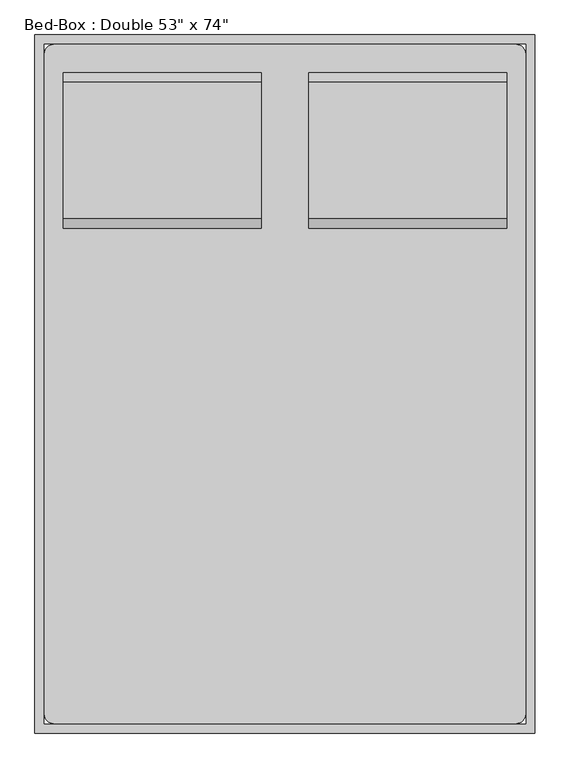
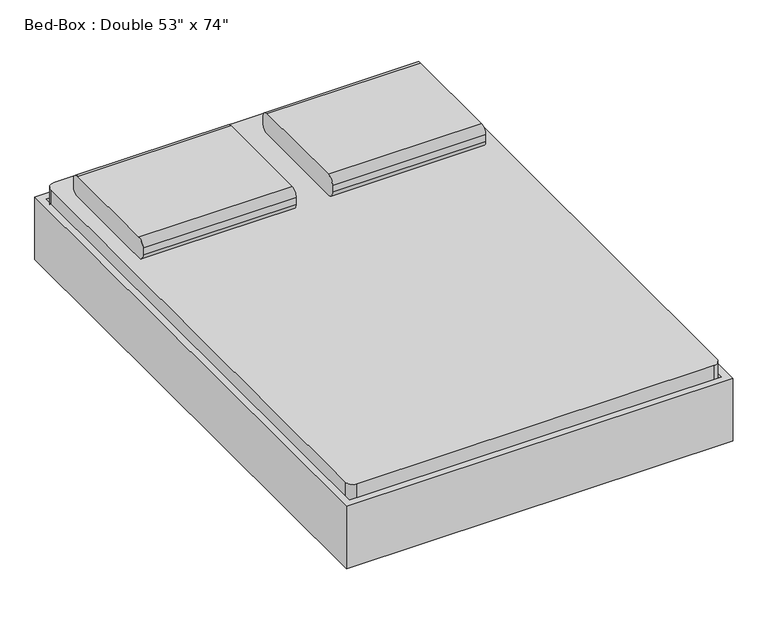
"""IFC4 building model written with IfcOpenShell, lengths in millimetres: furniture geometry."""

from ifc_helpers import new_model, si_unit, point, frame, frame_2d, origin, place, context, project, spatial, polyline, circle_curve, trimmed, segment, composite_curve, outline, extrude, source, transform, mapped, element, save
from ifc_brep_helpers import plane_surface, cylinder_surface, revolved_surface, advanced_brep


def furniture_b58f7881(model_context):
    return source(origin(), model_context, "Body", "SolidModel", [
        advanced_brep(
        [(-308.547541, -869.4295082, 196.85), (-308.547541, -869.4295082, 177.8), (-308.547541, -945.6295082, 177.8), (-308.547541, -945.6295082, 196.85), (-245.6113525, -869.4295082, 196.85), (-257.747541, -869.4295082, 177.8), (-257.747541, -945.6295082, 177.8), (-245.6113525, -945.6295082, 196.85), (-164.4115092, -869.4295082, 22.716374), (-181.6766725, -869.4295082, 14.6654962), (-181.6766725, -945.6295082, 14.6654962), (-164.4115092, -945.6295082, 22.716374), (-158.6564547, -869.4295082, 0.0), (-158.6564547, -869.4295082, 19.05), (-158.6564547, -945.6295082, 0.0), (-158.6564547, -945.6295082, 19.05), (-80.0439489, -869.4295082, 19.05), (-80.0439489, -869.4295082, 0.0), (-80.0439489, -945.6295082, 0.0), (-80.0439489, -945.6295082, 19.05), (-67.3439489, -869.4295082, 3.4029547), (-76.8689489, -869.4295082, 19.9007387), (-67.3439489, -945.6295082, 3.4029547), (-76.8689489, -945.6295082, 19.9007387), (-12.3513357, -869.4295082, 57.15), (-7.2469036, -869.4295082, 38.1), (-7.2469036, -945.6295082, 38.1), (-12.3513357, -945.6295082, 57.15), (690.6562537, -869.4295082, 57.15), (685.5518216, -869.4295082, 38.1), (685.5518216, -945.6295082, 38.1), (690.6562537, -945.6295082, 57.15), (755.1738669, -869.4295082, 19.9007387), (745.6488669, -869.4295082, 3.4029547), (745.6488669, -945.6295082, 3.4029547), (755.1738669, -945.6295082, 19.9007387), (758.3488669, -869.4295082, 0.0), (758.3488669, -869.4295082, 19.05), (758.3488669, -945.6295082, 0.0), (758.3488669, -945.6295082, 19.05), (836.9613728, -869.4295082, 19.05), (836.9613728, -869.4295082, 0.0), (836.9613728, -945.6295082, 0.0), (836.9613728, -945.6295082, 19.05), (859.9815906, -869.4295082, 14.6654962), (842.7164272, -869.4295082, 22.716374), (859.9815906, -945.6295082, 14.6654962), (842.7164272, -945.6295082, 22.716374), (923.9162705, -869.4295082, 196.85), (936.052459, -869.4295082, 177.8), (936.052459, -945.6295082, 177.8), (923.9162705, -945.6295082, 196.85), (986.852459, -869.4295082, 196.85), (986.852459, -945.6295082, 196.85), (986.852459, -945.6295082, 177.8), (986.852459, -869.4295082, 177.8)],
        [
            (0, 1),
            (1, 2),
            (2, 3),
            (3, 0),
            (0, 4),
            (4, 5),
            (5, 1),
            (5, 6),
            (6, 2),
            (6, 7),
            (7, 3),
            (7, 4),
            (4, 8),
            (8, 9),
            (9, 5),
            (9, 10),
            (10, 6),
            (10, 11),
            (11, 7),
            (11, 8),
            (12, 9, circle_curve(frame((-158.6564547, -869.4295082, 25.4), z_axis=(0.0, 1.0, 0.0), x_axis=(-0.906307787036663, 0.0, -0.4226182617406713)), 25.4)),
            (8, 13, circle_curve(frame((-158.6564547, -869.4295082, 25.4), z_axis=(0.0, -1.0, 0.0), x_axis=(-0.906307787036663, 0.0, -0.4226182617406713)), 6.35)),
            (13, 12),
            (14, 10, circle_curve(frame((-158.6564547, -945.6295082, 25.4), z_axis=(0.0, 1.0, 0.0), x_axis=(-0.906307787036663, 0.0, -0.4226182617406713)), 25.4)),
            (12, 14),
            (15, 11, circle_curve(frame((-158.6564547, -945.6295082, 25.4), z_axis=(0.0, 1.0, 0.0), x_axis=(-0.906307787036663, 0.0, -0.4226182617406713)), 6.35)),
            (14, 15),
            (15, 13),
            (13, 16),
            (16, 17),
            (17, 12),
            (17, 18),
            (18, 14),
            (18, 19),
            (19, 15),
            (19, 16),
            (20, 17, circle_curve(frame((-80.0439489, -869.4295082, 25.4), z_axis=(0.0, 1.0, 0.0), x_axis=(0.0, 0.0, -1.0)), 25.4)),
            (16, 21, circle_curve(frame((-80.0439489, -869.4295082, 25.4), z_axis=(0.0, -1.0, 0.0), x_axis=(0.0, 0.0, -1.0)), 6.35)),
            (21, 20),
            (22, 18, circle_curve(frame((-80.0439489, -945.6295082, 25.4), z_axis=(0.0, 1.0, 0.0), x_axis=(0.0, 0.0, -1.0)), 25.4)),
            (20, 22),
            (23, 19, circle_curve(frame((-80.0439489, -945.6295082, 25.4), z_axis=(0.0, 1.0, 0.0), x_axis=(0.0, 0.0, -1.0)), 6.35)),
            (22, 23),
            (23, 21),
            (21, 24),
            (24, 25),
            (25, 20),
            (25, 26),
            (26, 22),
            (26, 27),
            (27, 23),
            (27, 24),
            (24, 28),
            (28, 29),
            (29, 25),
            (29, 30),
            (30, 26),
            (30, 31),
            (31, 27),
            (31, 28),
            (28, 32),
            (32, 33),
            (33, 29),
            (33, 34),
            (34, 30),
            (34, 35),
            (35, 31),
            (35, 32),
            (36, 33, circle_curve(frame((758.3488669, -869.4295082, 25.4), z_axis=(0.0, 1.0, 0.0), x_axis=(-0.5000000000000479, 0.0, -0.866025403784411)), 25.4)),
            (32, 37, circle_curve(frame((758.3488669, -869.4295082, 25.4), z_axis=(0.0, -1.0, 0.0), x_axis=(-0.5000000000000479, 0.0, -0.866025403784411)), 6.35)),
            (37, 36),
            (38, 34, circle_curve(frame((758.3488669, -945.6295082, 25.4), z_axis=(0.0, 1.0, 0.0), x_axis=(-0.5000000000000479, 0.0, -0.866025403784411)), 25.4)),
            (36, 38),
            (39, 35, circle_curve(frame((758.3488669, -945.6295082, 25.4), z_axis=(0.0, 1.0, 0.0), x_axis=(-0.5000000000000479, 0.0, -0.866025403784411)), 6.35)),
            (38, 39),
            (39, 37),
            (37, 40),
            (40, 41),
            (41, 36),
            (41, 42),
            (42, 38),
            (42, 43),
            (43, 39),
            (43, 40),
            (44, 41, circle_curve(frame((836.9613728, -869.4295082, 25.4), z_axis=(0.0, 1.0, 0.0), x_axis=(0.0, 0.0, -1.0)), 25.4)),
            (40, 45, circle_curve(frame((836.9613728, -869.4295082, 25.4), z_axis=(0.0, -1.0, 0.0), x_axis=(0.0, 0.0, -1.0)), 6.35)),
            (45, 44),
            (46, 42, circle_curve(frame((836.9613728, -945.6295082, 25.4), z_axis=(0.0, 1.0, 0.0), x_axis=(0.0, 0.0, -1.0)), 25.4)),
            (44, 46),
            (47, 43, circle_curve(frame((836.9613728, -945.6295082, 25.4), z_axis=(0.0, 1.0, 0.0), x_axis=(0.0, 0.0, -1.0)), 6.35)),
            (46, 47),
            (47, 45),
            (45, 48),
            (48, 49),
            (49, 44),
            (49, 50),
            (50, 46),
            (50, 51),
            (51, 47),
            (51, 48),
            (52, 53),
            (53, 54),
            (54, 55),
            (55, 52),
            (48, 52),
            (55, 49),
            (54, 50),
            (53, 51),
        ],
        [
            plane_surface(frame((-308.547541, -1174.2295082, -127.5947323), z_axis=(-1.0, 0.0, 0.0), x_axis=(0.0, 1.0, 0.0))),
            plane_surface(frame((-308.547541, -869.4295082, 196.85), z_axis=(0.0, 1.0, 0.0), x_axis=(1.0, 0.0, 0.0))),
            plane_surface(frame((-308.547541, -869.4295082, 177.8), z_axis=(0.0, 0.0, -1.0), x_axis=(1.0, 0.0, 0.0))),
            plane_surface(frame((-308.547541, -945.6295082, 177.8), z_axis=(0.0, -1.0, 0.0), x_axis=(1.0, 0.0, 0.0))),
            plane_surface(frame((-308.547541, -945.6295082, 196.85), z_axis=(0.0, 0.0, 1.0), x_axis=(1.0, 0.0, 0.0))),
            plane_surface(frame((-245.6113525, -869.4295082, 196.85), z_axis=(0.0, 1.0, 0.0), x_axis=(0.422618261740671, 0.0, -0.9063077870366633))),
            plane_surface(frame((-257.747541, -869.4295082, 177.8), z_axis=(-0.9063077870366631, 0.0, -0.42261826174067113), x_axis=(0.42261826174067113, 0.0, -0.9063077870366631))),
            plane_surface(frame((-257.747541, -945.6295082, 177.8), z_axis=(0.0, -1.0, 0.0), x_axis=(0.42261826174067135, 0.0, -0.906307787036663))),
            plane_surface(frame((-245.6113525, -945.6295082, 196.85), z_axis=(0.9063077870366631, 0.0, 0.4226182617406713), x_axis=(0.4226182617406713, 0.0, -0.9063077870366631))),
            plane_surface(frame((-158.6564547, -869.4295082, 25.4), z_axis=(0.0, 1.0, 0.0), x_axis=(-0.906307787036663, 0.0, -0.4226182617406713))),
            cylinder_surface(frame((-158.6564547, -1174.2295082, 25.4), z_axis=(0.0, -1.0, 0.0), x_axis=(-0.906307787036663, 0.0, -0.4226182617406713)), 25.4),
            plane_surface(frame((-158.6564547, -945.6295082, 25.4), z_axis=(0.0, -1.0, 0.0), x_axis=(-0.906307787036663, 0.0, -0.4226182617406713))),
            revolved_surface(polyline([(-164.41150914768284, -945.6295082, 22.716374037946736), (-164.41150914768284, -869.4295082, 22.716374037946736)]), (-158.6564547, -1174.2295082, 25.4), (0.0, -1.0, 0.0)),
            plane_surface(frame((-158.6564547, -869.4295082, 19.05), z_axis=(0.0, 1.0, 0.0), x_axis=(1.0, 0.0, 0.0))),
            plane_surface(frame((-158.6564547, -869.4295082, 0.0), z_axis=(0.0, 0.0, -1.0), x_axis=(1.0, 0.0, 0.0))),
            plane_surface(frame((-158.6564547, -945.6295082, 0.0), z_axis=(0.0, -1.0, 0.0), x_axis=(1.0, 0.0, 0.0))),
            plane_surface(frame((-158.6564547, -945.6295082, 19.05), z_axis=(0.0, 0.0, 1.0), x_axis=(1.0, 0.0, 0.0))),
            plane_surface(frame((-80.0439489, -869.4295082, 25.4), z_axis=(0.0, 1.0, 0.0), x_axis=(0.0, 0.0, -1.0))),
            cylinder_surface(frame((-80.0439489, -1174.2295082, 25.4), z_axis=(0.0, -1.0, 0.0), x_axis=(0.0, 0.0, -1.0)), 25.4),
            plane_surface(frame((-80.0439489, -945.6295082, 25.4), z_axis=(0.0, -1.0, 0.0), x_axis=(0.0, 0.0, -1.0))),
            revolved_surface(polyline([(-80.0439489, -945.6295082, 19.049999999999997), (-80.0439489, -869.4295082, 19.049999999999997)]), (-80.0439489, -1174.2295082, 25.4), (0.0, -1.0, 0.0)),
            plane_surface(frame((-76.8689489, -869.4295082, 19.9007387), z_axis=(0.0, 1.0, 0.0), x_axis=(0.8660254037844785, 0.0, 0.499999999999931))),
            plane_surface(frame((-67.3439489, -869.4295082, 3.4029547), z_axis=(0.499999999999931, 0.0, -0.8660254037844785), x_axis=(0.8660254037844785, 0.0, 0.499999999999931))),
            plane_surface(frame((-67.3439489, -945.6295082, 3.4029547), z_axis=(0.0, -1.0, 0.0), x_axis=(0.8660254037844786, 0.0, 0.49999999999993094))),
            plane_surface(frame((-76.8689489, -945.6295082, 19.9007387), z_axis=(-0.4999999999999312, 0.0, 0.8660254037844785), x_axis=(0.8660254037844785, 0.0, 0.4999999999999312))),
            plane_surface(frame((-12.3513357, -869.4295082, 57.15), z_axis=(0.0, 1.0, 0.0), x_axis=(1.0, 0.0, 0.0))),
            plane_surface(frame((-7.2469036, -869.4295082, 38.1), z_axis=(0.0, 0.0, -1.0), x_axis=(1.0, 0.0, 0.0))),
            plane_surface(frame((-7.2469036, -945.6295082, 38.1), z_axis=(0.0, -1.0, 0.0), x_axis=(1.0, 0.0, 0.0))),
            plane_surface(frame((-12.3513357, -945.6295082, 57.15), z_axis=(0.0, 0.0, 1.0), x_axis=(1.0, 0.0, 0.0))),
            plane_surface(frame((690.6562537, -869.4295082, 57.15), z_axis=(0.0, 1.0, 0.0), x_axis=(0.8660254037844091, 0.0, -0.5000000000000514))),
            plane_surface(frame((685.5518216, -869.4295082, 38.1), z_axis=(-0.5000000000000502, 0.0, -0.8660254037844097), x_axis=(0.8660254037844097, 0.0, -0.5000000000000502))),
            plane_surface(frame((685.5518216, -945.6295082, 38.1), z_axis=(0.0, -1.0, 0.0), x_axis=(0.86602540378441, 0.0, -0.5000000000000498))),
            plane_surface(frame((690.6562537, -945.6295082, 57.15), z_axis=(0.5000000000000505, 0.0, 0.8660254037844095), x_axis=(0.8660254037844095, 0.0, -0.5000000000000505))),
            plane_surface(frame((758.3488669, -869.4295082, 25.4), z_axis=(0.0, 1.0000000000000002, 0.0), x_axis=(-0.500000000000048, 0.0, -0.8660254037844111))),
            cylinder_surface(frame((758.3488669, -1174.2295082, 25.4), z_axis=(0.0, -1.0, 0.0), x_axis=(-0.5000000000000479, 0.0, -0.866025403784411)), 25.4),
            plane_surface(frame((758.3488669, -945.6295082, 25.4), z_axis=(0.0, -1.0000000000000002, 0.0), x_axis=(-0.500000000000048, 0.0, -0.8660254037844111))),
            revolved_surface(polyline([(755.1738668999997, -945.6295082, 19.90073868596899), (755.1738668999997, -869.4295082, 19.90073868596899)]), (758.3488669, -1174.2295082, 25.4), (0.0, -1.0, 0.0)),
            plane_surface(frame((758.3488669, -869.4295082, 19.05), z_axis=(0.0, 1.0, 0.0), x_axis=(1.0, 0.0, 0.0))),
            plane_surface(frame((758.3488669, -869.4295082, 0.0), z_axis=(0.0, 0.0, -1.0), x_axis=(1.0, 0.0, 0.0))),
            plane_surface(frame((758.3488669, -945.6295082, 0.0), z_axis=(0.0, -1.0, 0.0), x_axis=(1.0, 0.0, 0.0))),
            plane_surface(frame((758.3488669, -945.6295082, 19.05), z_axis=(0.0, 0.0, 1.0), x_axis=(1.0, 0.0, 0.0))),
            plane_surface(frame((836.9613728, -869.4295082, 25.4), z_axis=(0.0, 1.0, 0.0), x_axis=(0.0, 0.0, -1.0))),
            cylinder_surface(frame((836.9613728, -1174.2295082, 25.4), z_axis=(0.0, -1.0, 0.0), x_axis=(0.0, 0.0, -1.0)), 25.4),
            plane_surface(frame((836.9613728, -945.6295082, 25.4), z_axis=(0.0, -1.0, 0.0), x_axis=(0.0, 0.0, -1.0))),
            revolved_surface(polyline([(836.9613728, -945.6295082, 19.049999999999997), (836.9613728, -869.4295082, 19.049999999999997)]), (836.9613728, -1174.2295082, 25.4), (0.0, -1.0, 0.0)),
            plane_surface(frame((842.7164272, -869.4295082, 22.716374), z_axis=(0.0, 1.0, 0.0), x_axis=(0.4226182617405411, 0.0, 0.9063077870367238))),
            plane_surface(frame((859.9815906, -869.4295082, 14.6654962), z_axis=(0.9063077870367237, 0.0, -0.42261826174054157), x_axis=(0.42261826174054157, 0.0, 0.9063077870367237))),
            plane_surface(frame((859.9815906, -945.6295082, 14.6654962), z_axis=(0.0, -1.0, 0.0), x_axis=(0.4226182617405412, 0.0, 0.9063077870367238))),
            plane_surface(frame((842.7164272, -945.6295082, 22.716374), z_axis=(-0.906307787036724, 0.0, 0.422618261740541), x_axis=(0.422618261740541, 0.0, 0.906307787036724))),
            plane_surface(frame((986.852459, -1174.2295082, -127.5947323), z_axis=(1.0, 0.0, 0.0), x_axis=(0.0, 1.0, 0.0))),
            plane_surface(frame((923.9162705, -869.4295082, 196.85), z_axis=(0.0, 1.0, 0.0), x_axis=(1.0, 0.0, 0.0))),
            plane_surface(frame((936.052459, -869.4295082, 177.8), z_axis=(0.0, 0.0, -1.0), x_axis=(1.0, 0.0, 0.0))),
            plane_surface(frame((936.052459, -945.6295082, 177.8), z_axis=(0.0, -1.0, 0.0), x_axis=(1.0, 0.0, 0.0))),
            plane_surface(frame((923.9162705, -945.6295082, 196.85), z_axis=(0.0, 0.0, 1.0), x_axis=(1.0, 0.0, 0.0))),
        ],
        [
            (0, [[1, 2, 3, 4]]),
            (1, [[-1, 5, 6, 7]]),
            (2, [[-2, -7, 8, 9]]),
            (3, [[-3, -9, 10, 11]]),
            (4, [[-4, -11, 12, -5]]),
            (5, [[-6, 13, 14, 15]]),
            (6, [[-8, -15, 16, 17]]),
            (7, [[-10, -17, 18, 19]]),
            (8, [[-12, -19, 20, -13]]),
            (9, [[21, -14, 22, 23]]),
            (10, [[24, -16, -21, 25]]),
            (11, [[26, -18, -24, 27]]),
            (12, [[-22, -20, -26, 28]]),
            (13, [[-23, 29, 30, 31]]),
            (14, [[-25, -31, 32, 33]]),
            (15, [[-27, -33, 34, 35]]),
            (16, [[-28, -35, 36, -29]]),
            (17, [[37, -30, 38, 39]]),
            (18, [[40, -32, -37, 41]]),
            (19, [[42, -34, -40, 43]]),
            (20, [[-38, -36, -42, 44]]),
            (21, [[-39, 45, 46, 47]]),
            (22, [[-41, -47, 48, 49]]),
            (23, [[-43, -49, 50, 51]]),
            (24, [[-44, -51, 52, -45]]),
            (25, [[-46, 53, 54, 55]]),
            (26, [[-48, -55, 56, 57]]),
            (27, [[-50, -57, 58, 59]]),
            (28, [[-52, -59, 60, -53]]),
            (29, [[-54, 61, 62, 63]]),
            (30, [[-56, -63, 64, 65]]),
            (31, [[-58, -65, 66, 67]]),
            (32, [[-60, -67, 68, -61]]),
            (33, [[69, -62, 70, 71]]),
            (34, [[72, -64, -69, 73]]),
            (35, [[74, -66, -72, 75]]),
            (36, [[-70, -68, -74, 76]]),
            (37, [[-71, 77, 78, 79]]),
            (38, [[-73, -79, 80, 81]]),
            (39, [[-75, -81, 82, 83]]),
            (40, [[-76, -83, 84, -77]]),
            (41, [[85, -78, 86, 87]]),
            (42, [[88, -80, -85, 89]]),
            (43, [[90, -82, -88, 91]]),
            (44, [[-86, -84, -90, 92]]),
            (45, [[-87, 93, 94, 95]]),
            (46, [[-89, -95, 96, 97]]),
            (47, [[-91, -97, 98, 99]]),
            (48, [[-92, -99, 100, -93]]),
            (49, [[101, 102, 103, 104]]),
            (50, [[-94, 105, -104, 106]]),
            (51, [[-96, -106, -103, 107]]),
            (52, [[-98, -107, -102, 108]]),
            (53, [[-100, -108, -101, -105]]),
        ],
    ),
        extrude(outline(composite_curve([segment(polyline([(-283.147541, 679.9704918), (961.452459, 679.9704918)]), True, "CONTINUOUS"), segment(trimmed(circle_curve(frame_2d((961.452459, 654.5704918)), 25.4), [point((961.452459, 679.9704918))], [point((986.852459, 654.5704918))], False, "CARTESIAN"), True, "CONTINUOUS"), segment(polyline([(986.852459, 654.5704918), (986.852459, -1123.4295082)]), True, "CONTINUOUS"), segment(trimmed(circle_curve(frame_2d((961.452459, -1123.4295082)), 25.4), [point((986.852459, -1123.4295082))], [point((961.452459, -1148.8295082))], False, "CARTESIAN"), True, "CONTINUOUS"), segment(polyline([(961.452459, -1148.8295082), (-283.147541, -1148.8295082)]), True, "CONTINUOUS"), segment(trimmed(circle_curve(frame_2d((-283.147541, -1123.4295082)), 25.4), [point((-283.147541, -1148.8295082))], [point((-308.547541, -1123.4295082))], False, "CARTESIAN"), True, "CONTINUOUS"), segment(polyline([(-308.547541, -1123.4295082), (-308.547541, 654.5704918)]), True, "CONTINUOUS"), segment(trimmed(circle_curve(frame_2d((-283.147541, 654.5704918)), 25.4), [point((-308.547541, 654.5704918))], [point((-283.147541, 679.9704918))], False, "CARTESIAN"), True, "CONTINUOUS")], self_intersect=False)), frame((0.0, 0.0, 203.2), z_axis=(0.0, 0.0, 1.0), x_axis=(1.0, 0.0, 0.0)), (0.0, 0.0, 1.0), 203.2),
        advanced_brep(
        [(-308.2231784, 451.3704918, 177.8), (-308.2231784, 375.1704918, 177.8), (-308.2231784, 375.1704918, 196.85), (-308.2231784, 451.3704918, 196.85), (-257.4231784, 451.3704918, 177.8), (-257.4231784, 375.1704918, 177.8), (-245.2869899, 375.1704918, 196.85), (-245.2869899, 451.3704918, 196.85), (-181.3523099, 451.3704918, 14.6654962), (-181.3523099, 375.1704918, 14.6654962), (-164.0871466, 375.1704918, 22.716374), (-164.0871466, 451.3704918, 22.716374), (-158.3320921, 375.1704918, 0.0), (-158.3320921, 451.3704918, 0.0), (-158.3320921, 375.1704918, 19.05), (-158.3320921, 451.3704918, 19.05), (-79.7195862, 451.3704918, 0.0), (-79.7195862, 375.1704918, 0.0), (-79.7195862, 375.1704918, 19.05), (-79.7195862, 451.3704918, 19.05), (-67.0195862, 375.1704918, 3.4029547), (-67.0195862, 451.3704918, 3.4029547), (-76.5445862, 375.1704918, 19.9007387), (-76.5445862, 451.3704918, 19.9007387), (-6.922541, 451.3704918, 38.1), (-6.922541, 375.1704918, 38.1), (-12.0269731, 375.1704918, 57.15), (-12.0269731, 451.3704918, 57.15), (685.5518216, 451.3704918, 38.1), (685.5518216, 375.1704918, 38.1), (690.6562537, 375.1704918, 57.15), (690.6562537, 451.3704918, 57.15), (745.6488669, 451.3704918, 3.4029547), (745.6488669, 375.1704918, 3.4029547), (755.1738669, 375.1704918, 19.9007387), (755.1738669, 451.3704918, 19.9007387), (758.3488669, 375.1704918, 0.0), (758.3488669, 451.3704918, 0.0), (758.3488669, 375.1704918, 19.05), (758.3488669, 451.3704918, 19.05), (836.9613728, 451.3704918, 0.0), (836.9613728, 375.1704918, 0.0), (836.9613728, 375.1704918, 19.05), (836.9613728, 451.3704918, 19.05), (859.9815906, 375.1704918, 14.6654962), (859.9815906, 451.3704918, 14.6654962), (842.7164272, 375.1704918, 22.716374), (842.7164272, 451.3704918, 22.716374), (936.052459, 451.3704918, 177.8), (936.052459, 375.1704918, 177.8), (923.9162705, 375.1704918, 196.85), (923.9162705, 451.3704918, 196.85), (986.852459, 451.3704918, 177.8), (986.852459, 451.3704918, 196.85), (986.852459, 375.1704918, 196.85), (986.852459, 375.1704918, 177.8)],
        [
            (0, 1),
            (1, 2),
            (2, 3),
            (3, 0),
            (0, 4),
            (4, 5),
            (5, 1),
            (5, 6),
            (6, 2),
            (6, 7),
            (7, 3),
            (7, 4),
            (4, 8),
            (8, 9),
            (9, 5),
            (9, 10),
            (10, 6),
            (10, 11),
            (11, 7),
            (11, 8),
            (12, 9, circle_curve(frame((-158.3320921, 375.1704918, 25.4), z_axis=(0.0, 1.0, 0.0), x_axis=(-0.9063077870366486, 0.0, -0.42261826174070233)), 25.4)),
            (8, 13, circle_curve(frame((-158.3320921, 451.3704918, 25.4), z_axis=(0.0, -1.0, 0.0), x_axis=(-0.9063077870366486, 0.0, -0.42261826174070233)), 25.4)),
            (13, 12),
            (14, 10, circle_curve(frame((-158.3320921, 375.1704918, 25.4), z_axis=(0.0, 1.0, 0.0), x_axis=(-0.9063077870366486, 0.0, -0.42261826174070233)), 6.35)),
            (12, 14),
            (15, 11, circle_curve(frame((-158.3320921, 451.3704918, 25.4), z_axis=(0.0, 1.0, 0.0), x_axis=(-0.9063077870366486, 0.0, -0.42261826174070233)), 6.35)),
            (14, 15),
            (15, 13),
            (13, 16),
            (16, 17),
            (17, 12),
            (17, 18),
            (18, 14),
            (18, 19),
            (19, 15),
            (19, 16),
            (20, 17, circle_curve(frame((-79.7195862, 375.1704918, 25.4), z_axis=(0.0, 1.0, 0.0), x_axis=(0.0, 0.0, -1.0)), 25.4)),
            (16, 21, circle_curve(frame((-79.7195862, 451.3704918, 25.4), z_axis=(0.0, -1.0, 0.0), x_axis=(0.0, 0.0, -1.0)), 25.4)),
            (21, 20),
            (22, 18, circle_curve(frame((-79.7195862, 375.1704918, 25.4), z_axis=(0.0, 1.0, 0.0), x_axis=(0.0, 0.0, -1.0)), 6.35)),
            (20, 22),
            (23, 19, circle_curve(frame((-79.7195862, 451.3704918, 25.4), z_axis=(0.0, 1.0, 0.0), x_axis=(0.0, 0.0, -1.0)), 6.35)),
            (22, 23),
            (23, 21),
            (21, 24),
            (24, 25),
            (25, 20),
            (25, 26),
            (26, 22),
            (26, 27),
            (27, 23),
            (27, 24),
            (24, 28),
            (28, 29),
            (29, 25),
            (29, 30),
            (30, 26),
            (30, 31),
            (31, 27),
            (31, 28),
            (28, 32),
            (32, 33),
            (33, 29),
            (33, 34),
            (34, 30),
            (34, 35),
            (35, 31),
            (35, 32),
            (36, 33, circle_curve(frame((758.3488669, 375.1704918, 25.4), z_axis=(0.0, 1.0, 0.0), x_axis=(-0.5000000000000463, 0.0, -0.8660254037844118)), 25.4)),
            (32, 37, circle_curve(frame((758.3488669, 451.3704918, 25.4), z_axis=(0.0, -1.0, 0.0), x_axis=(-0.5000000000000463, 0.0, -0.8660254037844118)), 25.4)),
            (37, 36),
            (38, 34, circle_curve(frame((758.3488669, 375.1704918, 25.4), z_axis=(0.0, 1.0, 0.0), x_axis=(-0.5000000000000463, 0.0, -0.8660254037844118)), 6.35)),
            (36, 38),
            (39, 35, circle_curve(frame((758.3488669, 451.3704918, 25.4), z_axis=(0.0, 1.0, 0.0), x_axis=(-0.5000000000000463, 0.0, -0.8660254037844118)), 6.35)),
            (38, 39),
            (39, 37),
            (37, 40),
            (40, 41),
            (41, 36),
            (41, 42),
            (42, 38),
            (42, 43),
            (43, 39),
            (43, 40),
            (44, 41, circle_curve(frame((836.9613728, 375.1704918, 25.4), z_axis=(0.0, 1.0, 0.0), x_axis=(0.0, 0.0, -1.0)), 25.4)),
            (40, 45, circle_curve(frame((836.9613728, 451.3704918, 25.4), z_axis=(0.0, -1.0, 0.0), x_axis=(0.0, 0.0, -1.0)), 25.4)),
            (45, 44),
            (46, 42, circle_curve(frame((836.9613728, 375.1704918, 25.4), z_axis=(0.0, 1.0, 0.0), x_axis=(0.0, 0.0, -1.0)), 6.35)),
            (44, 46),
            (47, 43, circle_curve(frame((836.9613728, 451.3704918, 25.4), z_axis=(0.0, 1.0, 0.0), x_axis=(0.0, 0.0, -1.0)), 6.35)),
            (46, 47),
            (47, 45),
            (45, 48),
            (48, 49),
            (49, 44),
            (49, 50),
            (50, 46),
            (50, 51),
            (51, 47),
            (51, 48),
            (52, 53),
            (53, 54),
            (54, 55),
            (55, 52),
            (48, 52),
            (55, 49),
            (54, 50),
            (53, 51),
        ],
        [
            plane_surface(frame((-308.2231784, 705.3704918, -152.9490627), z_axis=(-1.0, 0.0, 0.0), x_axis=(0.0, 1.0, 0.0))),
            plane_surface(frame((-308.2231784, 451.3704918, 177.8), z_axis=(0.0, 0.0, -1.0), x_axis=(1.0, 0.0, 0.0))),
            plane_surface(frame((-308.2231784, 375.1704918, 177.8), z_axis=(0.0, -1.0, 0.0), x_axis=(1.0, 0.0, 0.0))),
            plane_surface(frame((-308.2231784, 375.1704918, 196.85), z_axis=(0.0, 0.0, 1.0), x_axis=(1.0, 0.0, 0.0))),
            plane_surface(frame((-308.2231784, 451.3704918, 196.85), z_axis=(0.0, 1.0, 0.0), x_axis=(1.0, 0.0, 0.0))),
            plane_surface(frame((-257.4231784, 451.3704918, 177.8), z_axis=(-0.9063077870366488, 0.0, -0.42261826174070194), x_axis=(0.42261826174070194, 0.0, -0.9063077870366488))),
            plane_surface(frame((-257.4231784, 375.1704918, 177.8), z_axis=(0.0, -1.0, 0.0), x_axis=(0.42261826174070194, 0.0, -0.9063077870366488))),
            plane_surface(frame((-245.2869899, 375.1704918, 196.85), z_axis=(0.9063077870366487, 0.0, 0.4226182617407021), x_axis=(0.4226182617407021, 0.0, -0.9063077870366487))),
            plane_surface(frame((-245.2869899, 451.3704918, 196.85), z_axis=(0.0, 1.0, 0.0), x_axis=(0.4226182617407021, 0.0, -0.9063077870366487))),
            cylinder_surface(frame((-158.3320921, 705.3704918, 25.4), z_axis=(0.0, -1.0, 0.0), x_axis=(-0.9063077870366486, 0.0, -0.42261826174070233)), 25.4),
            plane_surface(frame((-158.3320921, 375.1704918, 25.4), z_axis=(0.0, -1.0, 0.0), x_axis=(-0.9063077870366486, 0.0, -0.42261826174070233))),
            revolved_surface(polyline([(-164.08714654768272, 375.1704918, 22.71637403794654), (-164.08714654768272, 451.3704918, 22.71637403794654)]), (-158.3320921, 705.3704918, 25.4), (0.0, -1.0, 0.0)),
            plane_surface(frame((-158.3320921, 451.3704918, 25.4), z_axis=(0.0, 1.0, 0.0), x_axis=(-0.9063077870366486, 0.0, -0.42261826174070233))),
            plane_surface(frame((-158.3320921, 451.3704918, 0.0), z_axis=(0.0, 0.0, -1.0), x_axis=(1.0, 0.0, 0.0))),
            plane_surface(frame((-158.3320921, 375.1704918, 0.0), z_axis=(0.0, -1.0, 0.0), x_axis=(1.0, 0.0, 0.0))),
            plane_surface(frame((-158.3320921, 375.1704918, 19.05), z_axis=(0.0, 0.0, 1.0), x_axis=(1.0, 0.0, 0.0))),
            plane_surface(frame((-158.3320921, 451.3704918, 19.05), z_axis=(0.0, 1.0, 0.0), x_axis=(1.0, 0.0, 0.0))),
            cylinder_surface(frame((-79.7195862, 705.3704918, 25.4), z_axis=(0.0, -1.0, 0.0), x_axis=(0.0, 0.0, -1.0)), 25.4),
            plane_surface(frame((-79.7195862, 375.1704918, 25.4), z_axis=(0.0, -1.0, 0.0), x_axis=(0.0, 0.0, -1.0))),
            revolved_surface(polyline([(-79.7195862, 375.1704918, 19.049999999999997), (-79.7195862, 451.3704918, 19.049999999999997)]), (-79.7195862, 705.3704918, 25.4), (0.0, -1.0, 0.0)),
            plane_surface(frame((-79.7195862, 451.3704918, 25.4), z_axis=(0.0, 1.0, 0.0), x_axis=(0.0, 0.0, -1.0))),
            plane_surface(frame((-67.0195862, 451.3704918, 3.4029547), z_axis=(0.4999999999998775, 0.0, -0.8660254037845094), x_axis=(0.8660254037845094, 0.0, 0.4999999999998775))),
            plane_surface(frame((-67.0195862, 375.1704918, 3.4029547), z_axis=(0.0, -1.0, 0.0), x_axis=(0.866025403784509, 0.0, 0.49999999999987826))),
            plane_surface(frame((-76.5445862, 375.1704918, 19.9007387), z_axis=(-0.49999999999987754, 0.0, 0.8660254037845093), x_axis=(0.8660254037845093, 0.0, 0.49999999999987754))),
            plane_surface(frame((-76.5445862, 451.3704918, 19.9007387), z_axis=(0.0, 1.0000000000000002, 0.0), x_axis=(0.8660254037845091, 0.0, 0.49999999999987815))),
            plane_surface(frame((-6.922541, 451.3704918, 38.1), z_axis=(0.0, 0.0, -1.0), x_axis=(1.0, 0.0, 0.0))),
            plane_surface(frame((-6.922541, 375.1704918, 38.1), z_axis=(0.0, -1.0, 0.0), x_axis=(1.0, 0.0, 0.0))),
            plane_surface(frame((-12.0269731, 375.1704918, 57.15), z_axis=(0.0, 0.0, 1.0), x_axis=(1.0, 0.0, 0.0))),
            plane_surface(frame((-12.0269731, 451.3704918, 57.15), z_axis=(0.0, 1.0, 0.0), x_axis=(1.0, 0.0, 0.0))),
            plane_surface(frame((685.5518216, 451.3704918, 38.1), z_axis=(-0.500000000000047, 0.0, -0.8660254037844116), x_axis=(0.8660254037844116, 0.0, -0.500000000000047))),
            plane_surface(frame((685.5518216, 375.1704918, 38.1), z_axis=(0.0, -1.0, 0.0), x_axis=(0.8660254037844122, 0.0, -0.5000000000000459))),
            plane_surface(frame((690.6562537, 375.1704918, 57.15), z_axis=(0.5000000000000461, 0.0, 0.8660254037844121), x_axis=(0.8660254037844121, 0.0, -0.5000000000000461))),
            plane_surface(frame((690.6562537, 451.3704918, 57.15), z_axis=(0.0, 1.0, 0.0), x_axis=(0.8660254037844127, 0.0, -0.500000000000045))),
            cylinder_surface(frame((758.3488669, 705.3704918, 25.4), z_axis=(0.0, -1.0, 0.0), x_axis=(-0.5000000000000463, 0.0, -0.8660254037844118)), 25.4),
            plane_surface(frame((758.3488669, 375.1704918, 25.4), z_axis=(0.0, -1.0000000000000002, 0.0), x_axis=(-0.5000000000000464, 0.0, -0.866025403784412))),
            revolved_surface(polyline([(755.1738668999997, 375.1704918, 19.90073868596898), (755.1738668999997, 451.3704918, 19.90073868596898)]), (758.3488669, 705.3704918, 25.4), (0.0, -1.0, 0.0)),
            plane_surface(frame((758.3488669, 451.3704918, 25.4), z_axis=(0.0, 1.0000000000000002, 0.0), x_axis=(-0.5000000000000464, 0.0, -0.866025403784412))),
            plane_surface(frame((758.3488669, 451.3704918, 0.0), z_axis=(0.0, 0.0, -1.0), x_axis=(1.0, 0.0, 0.0))),
            plane_surface(frame((758.3488669, 375.1704918, 0.0), z_axis=(0.0, -1.0, 0.0), x_axis=(1.0, 0.0, 0.0))),
            plane_surface(frame((758.3488669, 375.1704918, 19.05), z_axis=(0.0, 0.0, 1.0), x_axis=(1.0, 0.0, 0.0))),
            plane_surface(frame((758.3488669, 451.3704918, 19.05), z_axis=(0.0, 1.0, 0.0), x_axis=(1.0, 0.0, 0.0))),
            cylinder_surface(frame((836.9613728, 705.3704918, 25.4), z_axis=(0.0, -1.0, 0.0), x_axis=(0.0, 0.0, -1.0)), 25.4),
            plane_surface(frame((836.9613728, 375.1704918, 25.4), z_axis=(0.0, -1.0, 0.0), x_axis=(0.0, 0.0, -1.0))),
            revolved_surface(polyline([(836.9613728, 375.1704918, 19.049999999999997), (836.9613728, 451.3704918, 19.049999999999997)]), (836.9613728, 705.3704918, 25.4), (0.0, -1.0, 0.0)),
            plane_surface(frame((836.9613728, 451.3704918, 25.4), z_axis=(0.0, 1.0, 0.0), x_axis=(0.0, 0.0, -1.0))),
            plane_surface(frame((859.9815906, 451.3704918, 14.6654962), z_axis=(0.9063077870366797, 0.0, -0.42261826174063566), x_axis=(0.42261826174063566, 0.0, 0.9063077870366797))),
            plane_surface(frame((859.9815906, 375.1704918, 14.6654962), z_axis=(0.0, -1.0000000000000002, 0.0), x_axis=(0.4226182617406349, 0.0, 0.9063077870366801))),
            plane_surface(frame((842.7164272, 375.1704918, 22.716374), z_axis=(-0.9063077870366799, 0.0, 0.4226182617406354), x_axis=(0.4226182617406354, 0.0, 0.9063077870366799))),
            plane_surface(frame((842.7164272, 451.3704918, 22.716374), z_axis=(0.0, 1.0, 0.0), x_axis=(0.42261826174063555, 0.0, 0.9063077870366798))),
            plane_surface(frame((986.852459, 705.3704918, -152.9490627), z_axis=(1.0, 0.0, 0.0), x_axis=(0.0, 1.0, 0.0))),
            plane_surface(frame((936.052459, 451.3704918, 177.8), z_axis=(0.0, 0.0, -1.0), x_axis=(1.0, 0.0, 0.0))),
            plane_surface(frame((936.052459, 375.1704918, 177.8), z_axis=(0.0, -1.0, 0.0), x_axis=(1.0, 0.0, 0.0))),
            plane_surface(frame((923.9162705, 375.1704918, 196.85), z_axis=(0.0, 0.0, 1.0), x_axis=(1.0, 0.0, 0.0))),
            plane_surface(frame((923.9162705, 451.3704918, 196.85), z_axis=(0.0, 1.0, 0.0), x_axis=(1.0, 0.0, 0.0))),
        ],
        [
            (0, [[1, 2, 3, 4]]),
            (1, [[-1, 5, 6, 7]]),
            (2, [[-2, -7, 8, 9]]),
            (3, [[-3, -9, 10, 11]]),
            (4, [[-4, -11, 12, -5]]),
            (5, [[-6, 13, 14, 15]]),
            (6, [[-8, -15, 16, 17]]),
            (7, [[-10, -17, 18, 19]]),
            (8, [[-12, -19, 20, -13]]),
            (9, [[21, -14, 22, 23]]),
            (10, [[24, -16, -21, 25]]),
            (11, [[26, -18, -24, 27]]),
            (12, [[-22, -20, -26, 28]]),
            (13, [[-23, 29, 30, 31]]),
            (14, [[-25, -31, 32, 33]]),
            (15, [[-27, -33, 34, 35]]),
            (16, [[-28, -35, 36, -29]]),
            (17, [[37, -30, 38, 39]]),
            (18, [[40, -32, -37, 41]]),
            (19, [[42, -34, -40, 43]]),
            (20, [[-38, -36, -42, 44]]),
            (21, [[-39, 45, 46, 47]]),
            (22, [[-41, -47, 48, 49]]),
            (23, [[-43, -49, 50, 51]]),
            (24, [[-44, -51, 52, -45]]),
            (25, [[-46, 53, 54, 55]]),
            (26, [[-48, -55, 56, 57]]),
            (27, [[-50, -57, 58, 59]]),
            (28, [[-52, -59, 60, -53]]),
            (29, [[-54, 61, 62, 63]]),
            (30, [[-56, -63, 64, 65]]),
            (31, [[-58, -65, 66, 67]]),
            (32, [[-60, -67, 68, -61]]),
            (33, [[69, -62, 70, 71]]),
            (34, [[72, -64, -69, 73]]),
            (35, [[74, -66, -72, 75]]),
            (36, [[-70, -68, -74, 76]]),
            (37, [[-71, 77, 78, 79]]),
            (38, [[-73, -79, 80, 81]]),
            (39, [[-75, -81, 82, 83]]),
            (40, [[-76, -83, 84, -77]]),
            (41, [[85, -78, 86, 87]]),
            (42, [[88, -80, -85, 89]]),
            (43, [[90, -82, -88, 91]]),
            (44, [[-86, -84, -90, 92]]),
            (45, [[-87, 93, 94, 95]]),
            (46, [[-89, -95, 96, 97]]),
            (47, [[-91, -97, 98, 99]]),
            (48, [[-92, -99, 100, -93]]),
            (49, [[101, 102, 103, 104]]),
            (50, [[-94, 105, -104, 106]]),
            (51, [[-96, -106, -103, 107]]),
            (52, [[-98, -107, -102, 108]]),
            (53, [[-100, -108, -101, -105]]),
        ],
    ),
        extrude(outline(composite_curve([segment(polyline([(578.3704918, 406.4), (210.0704918, 406.4)]), True, "CONTINUOUS"), segment(trimmed(circle_curve(frame_2d((210.0704918, 431.8)), 25.4), [point((210.0704918, 406.4))], [point((184.6704918, 431.8))], False, "CARTESIAN"), True, "CONTINUOUS"), segment(polyline([(184.6704918, 431.8), (184.6704918, 457.2)]), True, "CONTINUOUS"), segment(trimmed(circle_curve(frame_2d((210.0704918, 457.2)), 25.4), [point((184.6704918, 457.2))], [point((210.0704918, 482.6))], False, "CARTESIAN"), True, "CONTINUOUS"), segment(polyline([(210.0704918, 482.6), (578.3704918, 482.6)]), True, "CONTINUOUS"), segment(trimmed(circle_curve(frame_2d((578.3704918, 457.2)), 25.4), [point((578.3704918, 482.6))], [point((603.7704918, 457.2))], False, "CARTESIAN"), True, "CONTINUOUS"), segment(polyline([(603.7704918, 457.2), (603.7704918, 431.8)]), True, "CONTINUOUS"), segment(trimmed(circle_curve(frame_2d((578.3704918, 431.8)), 25.4), [point((603.7704918, 431.8))], [point((578.3704918, 406.4))], False, "CARTESIAN"), True, "CONTINUOUS")], self_intersect=False)), frame((-257.747541, 0.0, 0.0), z_axis=(1.0, 0.0, 0.0), x_axis=(0.0, 1.0, 0.0)), (0.0, 0.0, 1.0), 533.4),
        extrude(outline(composite_curve([segment(polyline([(578.3704918, 406.4), (210.0704918, 406.4)]), True, "CONTINUOUS"), segment(trimmed(circle_curve(frame_2d((210.0704918, 431.8)), 25.4), [point((210.0704918, 406.4))], [point((184.6704918, 431.8))], False, "CARTESIAN"), True, "CONTINUOUS"), segment(polyline([(184.6704918, 431.8), (184.6704918, 457.2)]), True, "CONTINUOUS"), segment(trimmed(circle_curve(frame_2d((210.0704918, 457.2)), 25.4), [point((184.6704918, 457.2))], [point((210.0704918, 482.6))], False, "CARTESIAN"), True, "CONTINUOUS"), segment(polyline([(210.0704918, 482.6), (578.3704918, 482.6)]), True, "CONTINUOUS"), segment(trimmed(circle_curve(frame_2d((578.3704918, 457.2)), 25.4), [point((578.3704918, 482.6))], [point((603.7704918, 457.2))], False, "CARTESIAN"), True, "CONTINUOUS"), segment(polyline([(603.7704918, 457.2), (603.7704918, 431.8)]), True, "CONTINUOUS"), segment(trimmed(circle_curve(frame_2d((578.3704918, 431.8)), 25.4), [point((603.7704918, 431.8))], [point((578.3704918, 406.4))], False, "CARTESIAN"), True, "CONTINUOUS")], self_intersect=False)), frame((402.652459, 0.0, 0.0), z_axis=(1.0, 0.0, 0.0), x_axis=(0.0, 1.0, 0.0)), (0.0, 0.0, 1.0), 533.4),
        extrude(outline(polyline([(1012.252459, 705.3704918), (1012.252459, -1174.2295082), (-333.947541, -1174.2295082), (-333.947541, 705.3704918), (1012.252459, 705.3704918)]), holes=[polyline([(986.852459, 679.9704918), (-308.547541, 679.9704918), (-308.547541, -1148.8295082), (986.852459, -1148.8295082), (986.852459, 679.9704918)])]), frame((0.0, 0.0, 127.0), z_axis=(0.0, 0.0, 1.0), x_axis=(1.0, 0.0, 0.0)), (0.0, 0.0, 1.0), 228.6),
    ])


if __name__ == "__main__":
    model = new_model("IFC4")
    model_context = context("Model", 3, world=origin())
    ifc_project = project(units=[si_unit("LENGTHUNIT", "METRE", prefix="MILLI")], contexts=[model_context])
    site = spatial("IfcSite", under=ifc_project)
    building = spatial("IfcBuilding", under=site)
    placement = place(None, origin())
    furniture_shape = furniture_b58f7881(model_context)
    element("IfcFurniture", 1, ObjectType="Bed-Box : Double 53\" x 74\"", at=placement, inside=building, context=model_context, shape_type="MappedRepresentation", body=[
        mapped(furniture_shape, transform((0.0, 0.0, 0.0), x_axis=(1.0, 0.0, 0.0), y_axis=(0.0, 1.0, 0.0), z_axis=(0.0, 0.0, 1.0))),
    ])
    save(model, "model.ifc")

# Revit data of these elements
# Type "Bed-Box : Double 53\" x 74\""
#   Assembly Code = "E2020200"
#   Length = 6.166667 ft
#   Width = 4.416667 ft
#   Frame Material = Birch
#   Mattress Material = Linen, White
#   Default Elevation = 0
# Element 1 (IfcFurniture, "Bed-Box : Double 53\" x 74\"")
#   Materials on its faces: "Birch", "Linen, White"
# Materials
#   "Birch": class "Wood", colour RGB 224 178 126, transparency 0, Description = "Betula Alleghaniensis", Cost = 0
#   "Linen, White": class "Textile", colour RGB 247 247 239, transparency 0, Description = "Linen, white", Cost = 0
